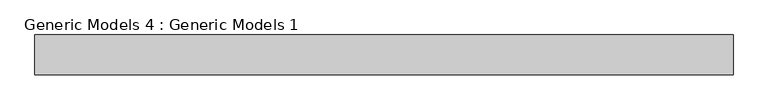
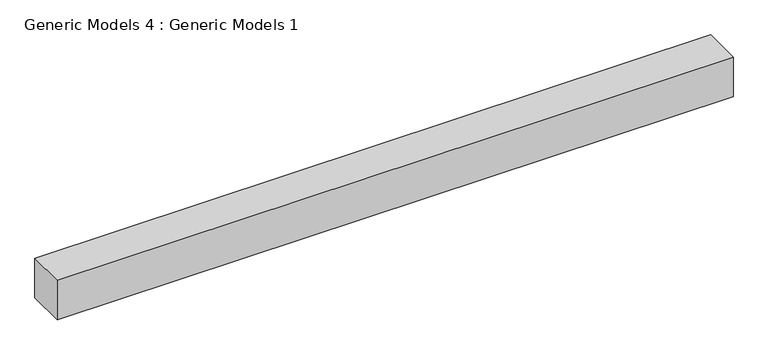
"""IFC4 building model written with IfcOpenShell, lengths in millimetres: proxy geometry, Generic Models 4 : Generic Models 1."""

from ifc_helpers import new_model, si_unit, frame, origin, place, context, project, spatial, polyline, outline, extrude, source, transform, mapped, element, save


def generic_models_4_generic_models_1_d4ed459b(model_context):
    return source(origin(), model_context, "Body", "SweptSolid", [
        extrude(outline(polyline([(-12111.4647504, -5734.4090801), (-17444.0507021, -5734.4090801), (-17444.0507021, -5429.6090801), (-12111.4647504, -5429.6090801), (-12111.4647504, -5734.4090801)])), frame((0.0, 0.0, 5572.0), z_axis=(0.0, 0.0, 1.0), x_axis=(1.0, 0.0, 0.0)), (0.0, 0.0, 1.0), 330.2),
    ])


if __name__ == "__main__":
    model = new_model("IFC4")
    model_context = context("Model", 3, world=origin())
    ifc_project = project(units=[si_unit("LENGTHUNIT", "METRE", prefix="MILLI")], contexts=[model_context])
    site = spatial("IfcSite", under=ifc_project)
    building = spatial("IfcBuilding", under=site)
    placement = place(None, origin())
    generic_models_4_generic_models_1_shape = generic_models_4_generic_models_1_d4ed459b(model_context)
    element("IfcBuildingElementProxy", 1, Name="Generic Models 4 : Generic Models 1", ObjectType="Generic Models 4 : Generic Models 1", at=placement, inside=building, context=model_context, shape_type="MappedRepresentation", body=[
        mapped(generic_models_4_generic_models_1_shape, transform((0.0, 0.0, 0.0), x_axis=(1.0, 0.0, 0.0), y_axis=(0.0, 1.0, 0.0), z_axis=(0.0, 0.0, 1.0))),
    ])
    save(model, "model.ifc")
